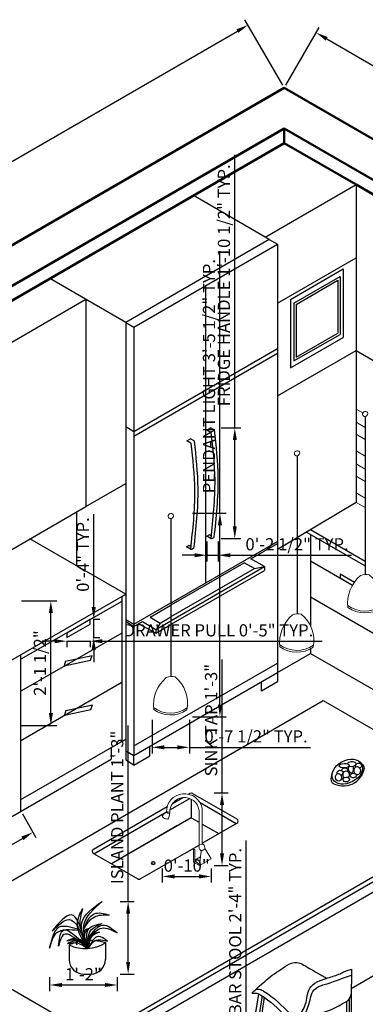
# Model space of a CAD drawing. Units: inches. Extents: x 5770 to 11891, y 3254 to 6808.
# Tile 3 of 15: x 5905 to 5976, y 3361 to 3563. Entities that reach past the tile are written whole.
import ezdxf

# ---------------------------------------------------------------- set-up
doc = ezdxf.new("R2010")
doc.units = ezdxf.units.IN
for name, color, linetype, lineweight in [('A-ANNO-DIMS', 2, 'Continuous', 18), ('A-FLOR-FIXT', 9, 'Continuous', 18), ('A-FURN', 8, 'Continuous', 25), ('A-WALL', 7, 'Continuous', 50), ('A-WALL-PATT', 8, 'Continuous', 13), ('E-LITE', 3, 'Continuous', 18)]:
    doc.layers.add(name, color=color, linetype=linetype, lineweight=lineweight)
doc.styles.get("Standard").update_dxf_attribs({"font": 'arial.ttf'})
doc.dimstyles.new('ISO-25', dxfattribs={"dimtxt": 2.5, "dimasz": 2.5, "dimexe": 1.25, "dimexo": 0.625, "dimtad": 1, "dimdec": 0, "dimlunit": 3, "dimtxsty": 'Standard', "dimcen": 2.5, "dimadec": 0, "dimazin": 0, "dimtfac": 1, "dimtdec": 0, "dimtmove": 0, "dimatfit": 3, "dimfxl": 1, "dimarcsym": 0})

# ---------------------------------------------------------------- blocks, each defined once
blk = doc.blocks.new('*D4')
at = {"layer": 'A-ANNO-DIMS', "color": 0, "lineweight": -2, "transparency": 16777216}
for p, q in [((5905.64, 3400.14), (5908.43, 3395.3)), ((5884.29, 3382.81), (5905.64, 3395.14)), ((5879.96, 3385.31), (5882.75, 3380.47))]:
    blk.add_line(p, q, dxfattribs=at)
at = {"layer": 'A-ANNO-DIMS', "color": 0, "transparency": 16777216}
for points in [[(5905.43, 3395.5), (5905.85, 3394.77), (5907.81, 3396.39)], [(5884.08, 3383.17), (5884.5, 3382.45), (5882.12, 3381.56)]]:
    blk.add_solid(points, dxfattribs=at)
at = {"layer": 'Defpoints', "color": 0, "transparency": 16777216}
for p in [(5905.33, 3400.68), (5907.81, 3396.39), (5879.65, 3385.85)]:
    blk.add_point(p, dxfattribs=at)
at = {"layer": 'A-ANNO-DIMS', "color": 0, "transparency": 16777216, "insert": (5894.02, 3390.62), "char_height": 2.5, "attachment_point": 5, "rotation": 30}
blk.add_mtext('2\'-6"', dxfattribs=at)
blk = doc.blocks.new('*D5')
at = {"layer": 'A-ANNO-DIMS', "color": 0, "lineweight": -2, "transparency": 16777216}
for p, q in [((5959, 3549.37), (5951.25, 3562.79)), ((5780.84, 3462.96), (5949.71, 3560.46)), ((5785.8, 3449.37), (5778.05, 3462.79))]:
    blk.add_line(p, q, dxfattribs=at)
at = {"layer": 'A-ANNO-DIMS', "color": 0, "transparency": 16777216}
for points in [[(5949.5, 3560.82), (5949.92, 3560.1), (5951.88, 3561.71)], [(5780.63, 3463.32), (5781.05, 3462.6), (5778.67, 3461.71)]]:
    blk.add_solid(points, dxfattribs=at)
at = {"layer": 'Defpoints', "color": 0, "transparency": 16777216}
for p in [(5951.88, 3561.71), (5959.31, 3548.83), (5786.11, 3448.83)]:
    blk.add_point(p, dxfattribs=at)
at = {"layer": 'A-ANNO-DIMS', "color": 0, "transparency": 16777216, "insert": (5864.32, 3513.36), "char_height": 2.5, "attachment_point": 5, "rotation": 30}
blk.add_mtext('16\'-8"', dxfattribs=at)
blk = doc.blocks.new('*D7')
at = {"layer": 'A-ANNO-DIMS', "color": 0, "lineweight": -2, "transparency": 16777216}
for p, q in [((5959.63, 3549.37), (5966.46, 3561.21)), ((5968, 3558.88), (6136.88, 3461.38)), ((6132.83, 3449.37), (6139.67, 3461.21))]:
    blk.add_line(p, q, dxfattribs=at)
at = {"layer": 'A-ANNO-DIMS', "color": 0, "transparency": 16777216}
for points in [[(5968.21, 3559.24), (5967.79, 3558.51), (5965.84, 3560.13)], [(6137.08, 3461.74), (6136.67, 3461.01), (6139.04, 3460.13)]]:
    blk.add_solid(points, dxfattribs=at)
at = {"layer": 'Defpoints', "color": 0, "transparency": 16777216}
for p in [(5959.31, 3548.83), (6139.04, 3460.13), (6132.52, 3448.83)]:
    blk.add_point(p, dxfattribs=at)
at = {"layer": 'A-ANNO-DIMS', "color": 0, "transparency": 16777216, "insert": (6061.62, 3507.02), "char_height": 2.5, "attachment_point": 5, "rotation": 330}
blk.add_mtext('16\'-8"', dxfattribs=at)
blk = doc.blocks.new('BULB')
for p, q in [((5936.06, 3465.13), (5936.06, 3432.77)), ((5936.16, 3465.15), (5936.16, 3432.77)), ((5936.06, 3432.77), (5936.16, 3432.77))]:
    blk.add_line(p, q)
for centre, radius, start, end in [((5939.83, 3426.9), 7.34, 129.7305, 187.2511), ((5936.2, 3430.31), 2.47, 73.0296, 115.4036), ((5932.63, 3427.32), 6.86, 348.0802, 51.2884), ((5936.01, 3431.26), 5.99, 234.2354, 304.5754), ((5935.99, 3430.88), 5.99, 234.9311, 303.9006)]:
    blk.add_arc(centre, radius, start, end)
blk.add_ellipse((5936.06, 3465.64), major_axis=(-0.492, -0.284), ratio=0.878374)
blk = doc.blocks.new('CHAIR')
for p, q in [((5928.22, 3348.4), (5925.54, 3331.45)), ((5928.97, 3347.97), (5926.27, 3331.03)), ((5929.39, 3347.7), (5926.87, 3331.3)), ((5946.78, 3347.31), (5946.81, 3331.7)), ((5947.21, 3348.3), (5947.24, 3331.95)), ((5946.25, 3346.87), (5946.28, 3331.94)), ((5935.16, 3343.21), (5935.19, 3327.16)), ((5935.65, 3343.13), (5935.69, 3326.87)), ((5936.61, 3343.23), (5936.64, 3327.43)), ((5936.93, 3343.31), (5936.93, 3335.67)), ((5937.63, 3343.48), (5937.63, 3336.08)), ((5927.75, 3337.02), (5935.16, 3341.28)), ((5937.62, 3341.89), (5946.27, 3336.9)), ((5937.62, 3341.39), (5946.27, 3336.4)), ((5927.68, 3336.56), (5935.16, 3340.78)), ((5935.18, 3331.68), (5927.6, 3336.05)), ((5935.18, 3332.18), (5927.67, 3336.51)), ((5936.63, 3335.85), (5936.93, 3335.67)), ((5946.27, 3336.9), (5936.64, 3331.34)), ((5946.27, 3336.4), (5936.64, 3330.84)), ((5937.63, 3336.08), (5936.93, 3335.67)), ((5925.54, 3331.45), (5926.27, 3331.03)), ((5926.27, 3331.03), (5926.87, 3331.3)), ((5946.28, 3331.94), (5946.75, 3331.67)), ((5946.75, 3331.67), (5947.24, 3331.95)), ((5935.69, 3326.87), (5935.19, 3327.16)), ((5935.69, 3326.87), (5936.64, 3327.43))]:
    blk.add_line(p, q)
blk.add_arc((5935.85, 3351.36), 3.39, 67.7359, 118.7768)
for points, knots in [([(5926.85, 3348.57), (5927.14, 3348.84), (5927.44, 3349.11), (5927.74, 3349.38), (5928.67, 3350.23), (5930.69, 3352.07), (5932.98, 3353.56), (5934.22, 3354.33)], [-1.200535, -1.200535, -1.200535, -1.200535, 0, 0, 0, 3.797995, 8.17369, 8.17369, 8.17369, 8.17369]), ([(5937.14, 3354.49), (5938.17, 3353.9), (5939.86, 3352.92), (5941.54, 3351.95), (5942.19, 3351.57)], [1.567957, 1.567957, 1.567957, 1.567957, 5.157778, 7.408601, 7.408601, 7.408601, 7.408601]), ([(5940.89, 3351.1), (5941.41, 3351.3), (5942.76, 3351.79), (5944.67, 3352.3), (5946.17, 3353.17), (5946.99, 3353.38), (5947.3, 3353.46)], [0, 0, 0, 0, 1.664278, 4.310629, 5.889247, 6.833724, 6.833724, 6.833724, 6.833724]), ([(5947.3, 3353.46), (5947.28, 3352.49), (5947.26, 3351.53), (5947.25, 3350.57), (5947.24, 3350.2), (5947.23, 3349.82), (5947.23, 3349.45), (5947.22, 3349.07), (5947.21, 3348.69), (5947.21, 3348.3)], [0, 0, 0, 0, 2.886502, 2.886502, 2.886502, 4.003886, 4.003886, 4.003886, 5.15459, 5.15459, 5.15459, 5.15459]), ([(5934.12, 3343.4), (5934.38, 3343.35), (5934.65, 3343.3), (5934.92, 3343.25), (5935.52, 3343.14), (5936.61, 3342.93), (5938.16, 3344.68), (5938.85, 3347.35), (5939.3, 3349.5), (5941.12, 3350.13), (5941.47, 3350.25), (5941.87, 3350.35), (5942.28, 3350.46), (5944.02, 3351.01), (5945.63, 3351.73), (5947.28, 3352.25)], [-0.758098, -0.758098, -0.758098, -0.758098, 0, 0, 0, 1.699756, 3.089131, 6.324639, 10.056959, 10.056959, 10.056959, 10.772274, 10.772274, 10.772274, 13.697346, 13.697346, 13.697346, 13.697346]), ([(5927.74, 3349.38), (5928, 3349.38), (5928.54, 3349.38), (5931.15, 3347.89), (5933.07, 3346.01), (5934.69, 3344.22)], [0, 0, 0, 0, 0.763361, 1.613257, 8.813397, 8.813397, 8.813397, 8.813397]), ([(5934.69, 3344.22), (5935.29, 3344.11), (5936.38, 3343.91), (5937.93, 3345.66), (5938.13, 3348.59), (5939.07, 3350.47), (5940.89, 3351.1)], [0, 0, 0, 0, 1.699756, 3.089131, 6.324639, 10.056959, 10.056959, 10.056959, 10.056959]), ([(5926.85, 3348.57), (5926.95, 3348.57), (5927.05, 3348.57), (5927.15, 3348.57), (5927.4, 3348.57), (5927.95, 3348.58), (5930.42, 3347.16), (5932.26, 3345.42), (5933.78, 3343.76), (5933.78, 3343.76), (5933.79, 3343.75), (5933.79, 3343.75), (5933.9, 3343.63), (5934.01, 3343.51), (5934.12, 3343.4)], [-0.293735, -0.293735, -0.293735, -0.293735, 0, 0, 0, 0.763361, 1.613257, 8.34273, 8.34273, 8.34273, 8.363036, 8.363036, 8.363036, 8.838355, 8.838355, 8.838355, 8.838355]), ([(5946.61, 3347.1), (5946.8, 3347.33), (5947.08, 3347.7), (5947.18, 3348.14), (5947.21, 3348.3)], [0, 0, 0, 0, 0.871891, 1.360739, 1.360739, 1.360739, 1.360739]), ([(5936.62, 3343.23), (5938.95, 3343.8), (5942.47, 3344.66), (5945.58, 3346.46), (5946.61, 3347.1)], [0, 0, 0, 0, 7.14919, 10.770772, 10.770772, 10.770772, 10.770772])]:
    blk.add_open_spline(points, degree=3, knots=knots)
blk = doc.blocks.new('TRESSS')
for p, q in [((5918.96, 3379.77), (5918.96, 3376.79)), ((5926.38, 3380.23), (5926.38, 3376.79)), ((5921.96, 3373.79), (5923.38, 3373.79))]:
    blk.add_line(p, q)
for centre, radius, start, end in [((5922.25, 3386.77), 7.74, 244.7929, 302.2014), ((5923.32, 3369.33), 11.31, 105.7826, 112.667), ((5923.32, 3369.33), 11.31, 101.3715, 102.257), ((5923.32, 3369.33), 11.31, 97.2364, 100.0777), ((5923.32, 3369.33), 11.31, 95.7662, 96.2014), ((5923.32, 3369.33), 11.31, 93.4301, 94.7766), ((5923.32, 3369.33), 11.31, 91.9955, 92.4941), ((5923.32, 3369.33), 11.31, 87.7241, 90.8189), ((5923.32, 3369.33), 11.31, 74.3273, 85.6124), ((5921.96, 3376.79), 3, 180, 270), ((5923.38, 3376.79), 3, 270, 0)]:
    blk.add_arc(centre, radius, start, end)
for points, knots in [([(5922.88, 3379.24), (5922.06, 3381.02), (5920.29, 3384.86), (5923.81, 3387.34), (5925.71, 3388.67)], [0, 0, 0, 0, 5.212698, 11.249377, 11.249377, 11.249377, 11.249377]), ([(5922.91, 3379.07), (5922.32, 3380.72), (5920.97, 3384.45), (5924.01, 3387.16), (5925.71, 3388.67)], [0, 0, 0, 0, 4.839765, 10.954456, 10.954456, 10.954456, 10.954456]), ([(5922.24, 3380.03), (5921.48, 3382.94), (5920.14, 3388.11), (5916.88, 3384.3), (5915.46, 3382.64)], [0, 0, 0, 0, 6.552433, 11.64556, 11.64556, 11.64556, 11.64556]), ([(5922.91, 3379.07), (5921.72, 3380.76), (5919.84, 3383.44), (5921.22, 3386.24), (5921.72, 3387.26)], [0, 0, 0, 0, 5.617277, 8.85563, 8.85563, 8.85563, 8.85563]), ([(5921.72, 3387.26), (5921.48, 3386.43), (5920.66, 3383.65), (5921.98, 3380.96), (5922.91, 3379.07)], [0, 0, 0, 0, 2.537454, 8.507618, 8.507618, 8.507618, 8.507618]), ([(5921.92, 3382.97), (5922.48, 3384.35), (5923.51, 3386.85), (5926.04, 3386.21), (5927.18, 3385.92)], [0, 0, 0, 0, 3.839673, 6.955686, 6.955686, 6.955686, 6.955686]), ([(5921.92, 3382.97), (5922.54, 3383.98), (5923.76, 3385.95), (5926.07, 3385.95), (5927.21, 3385.95)], [0, 0, 0, 0, 3.288518, 6.475213, 6.475213, 6.475213, 6.475213]), ([(5920.76, 3382.98), (5919.3, 3383.41), (5916.09, 3384.35), (5915.36, 3380.97), (5914.96, 3379.13)], [0, 0, 0, 0, 3.883772, 8.550412, 8.550412, 8.550412, 8.550412]), ([(5915.46, 3382.64), (5916.71, 3383.81), (5919.72, 3386.62), (5921.31, 3382.46), (5922.24, 3380.03)], [0, 0, 0, 0, 4.185411, 10.092894, 10.092894, 10.092894, 10.092894]), ([(5916.79, 3379.52), (5916.94, 3380.81), (5917.37, 3384.72), (5920.69, 3381.33), (5922.91, 3379.07)], [0, 0, 0, 0, 3.163863, 9.594114, 9.594114, 9.594114, 9.594114]), ([(5922.91, 3379.07), (5922.6, 3380.67), (5922.08, 3383.42), (5924.67, 3383.94), (5925.75, 3384.16)], [0, 0, 0, 0, 4.062167, 6.948759, 6.948759, 6.948759, 6.948759]), ([(5922.91, 3379.07), (5922.8, 3380.43), (5922.61, 3382.85), (5924.79, 3383.76), (5925.75, 3384.16)], [0, 0, 0, 0, 3.635219, 6.466255, 6.466255, 6.466255, 6.466255]), ([(5922.84, 3381.05), (5923.79, 3382.41), (5925.51, 3384.89), (5927.79, 3383.08), (5928.82, 3382.27)], [0, 0, 0, 0, 4.102984, 7.457094, 7.457094, 7.457094, 7.457094]), ([(5914.96, 3379.13), (5915.31, 3380.38), (5916.1, 3383.22), (5919.13, 3382.94), (5920.82, 3382.78)], [0, 0, 0, 0, 3.485265, 7.886828, 7.886828, 7.886828, 7.886828]), ([(5922.91, 3379.07), (5922.38, 3379.46), (5920.92, 3380.53), (5917.69, 3383.1), (5917.06, 3380.58), (5916.79, 3379.52)], [0, 0, 0, 0, 2.120674, 5.789324, 8.421631, 8.421631, 8.421631, 8.421631]), ([(5922.12, 3381.54), (5922.06, 3382.04), (5921.96, 3382.93), (5922.8, 3383.14), (5923.16, 3383.23)], [0, 0, 0, 0, 1.291281, 2.286027, 2.286027, 2.286027, 2.286027]), ([(5922.12, 3381.54), (5922.16, 3381.86), (5922.24, 3382.56), (5922.82, 3382.98), (5923.13, 3383.21)], [0, 0, 0, 0, 0.924204, 2.027617, 2.027617, 2.027617, 2.027617]), ([(5922.83, 3379.73), (5922.89, 3380.49), (5923, 3381.98), (5924.46, 3382.25), (5925.18, 3382.38)], [0, 0, 0, 0, 2.030096, 3.981846, 3.981846, 3.981846, 3.981846]), ([(5922.84, 3381.05), (5923.74, 3382.06), (5925.45, 3383.98), (5927.73, 3382.82), (5928.82, 3382.27)], [0, 0, 0, 0, 3.572941, 6.853548, 6.853548, 6.853548, 6.853548]), ([(5925.18, 3382.38), (5924.62, 3382.18), (5923.17, 3381.66), (5923.01, 3380.06), (5922.91, 3379.07)], [0, 0, 0, 0, 1.667038, 4.343126, 4.343126, 4.343126, 4.343126]), ([(5926.85, 3380.54), (5926.17, 3381.04), (5924.49, 3382.28), (5923.5, 3380.26), (5922.91, 3379.07)], [0, 0, 0, 0, 2.158738, 5.324445, 5.324445, 5.324445, 5.324445]), ([(5922.91, 3379.07), (5921.86, 3380.12), (5920.47, 3381.51), (5918.89, 3380.76), (5918.5, 3380.58)], [0, 0, 0, 0, 3.794821, 5.006614, 5.006614, 5.006614, 5.006614]), ([(5918.5, 3380.58), (5919.08, 3380.73), (5920.75, 3381.19), (5922.06, 3379.91), (5922.91, 3379.07)], [0, 0, 0, 0, 1.705074, 4.953728, 4.953728, 4.953728, 4.953728]), ([(5922.88, 3379.24), (5921.84, 3379.97), (5920.43, 3380.97), (5919.01, 3380.24), (5918.63, 3380.04)], [0, 0, 0, 0, 3.345341, 4.589329, 4.589329, 4.589329, 4.589329]), ([(5918.63, 3380.04), (5919.18, 3380.16), (5920.66, 3380.46), (5921.93, 3379.59), (5922.73, 3379.05)], [0, 0, 0, 0, 1.657681, 4.37303, 4.37303, 4.37303, 4.37303]), ([(5921.77, 3380.76), (5921.25, 3380.8), (5920.39, 3380.88), (5920.47, 3380.09), (5920.51, 3379.78)], [0, 0, 0, 0, 1.233849, 2.023752, 2.023752, 2.023752, 2.023752]), ([(5920.51, 3379.78), (5920.55, 3380.07), (5920.64, 3380.75), (5921.36, 3380.75), (5921.77, 3380.76)], [0, 0, 0, 0, 0.771667, 1.829769, 1.829769, 1.829769, 1.829769]), ([(5922.91, 3379.07), (5923.3, 3379.71), (5924.18, 3381.18), (5925.9, 3380.77), (5926.85, 3380.54)], [0, 0, 0, 0, 2.068412, 4.678786, 4.678786, 4.678786, 4.678786])]:
    blk.add_open_spline(points, degree=3, knots=knots)
blk = doc.blocks.new('*U16')
blk.add_circle((0, 0), 0.0159)
blk = doc.blocks.new('*U17')
at = {"layer": 'A-FURN', "color": 0, "linetype": 'ByBlock', "lineweight": -2, "transparency": 16777216}
for p, rotation in [((5932.23, 3390.22), 60), ((5932.24, 3389.96), 120), ((5932.47, 3389.82), 180), ((5932.7, 3390.23), 300), ((5932.7, 3389.96), 240)]:
    blk.add_blockref('*U16', p, dxfattribs=dict(at, rotation=rotation))
blk.add_blockref('*U16', (5932.47, 3390.36), dxfattribs=at)
blk = doc.blocks.new('TAP')
for p, q in [((5944.63, 3392.4), (5944.63, 3399.73)), ((5945.29, 3392.74), (5945.29, 3400.08)), ((5943.52, 3391.55), (5943.52, 3389.04)), ((5943.74, 3391.55), (5943.74, 3389.31)), ((5945.92, 3391.77), (5945.06, 3391.28)), ((5947.11, 3389.71), (5945.92, 3391.77)), ((5943.74, 3389.47), (5944.93, 3390.16)), ((5944.74, 3388.34), (5945.06, 3391.28)), ((5944.74, 3388.34), (5947.11, 3389.71)), ((5943.52, 3389.04), (5944.74, 3388.34)), ((5943.74, 3389.31), (5944.74, 3388.53))]:
    blk.add_line(p, q)
for centre, radius, start, end in [((5941.65, 3399.35), 3.7, 11.3324, 180.9911), ((5941.64, 3399.27), 3.02, 8.7526, 183.9319), ((5943.63, 3391.55), 0.111, 0, 180)]:
    blk.add_arc(centre, radius, start, end)
blk.add_ellipse((5938.29, 3399.19), major_axis=(-0.334, 0.124), ratio=0.36367)
for points, knots in [([(5937.95, 3399.3), (5937.78, 3399.2), (5937.42, 3399), (5937.21, 3398.66), (5937.11, 3398.48)], [0, 0, 0, 0, 0.588521, 1.1885, 1.1885, 1.1885, 1.1885]), ([(5937.11, 3398.48), (5937.18, 3398.34), (5937.38, 3397.9), (5937.89, 3397.88), (5938.22, 3397.87)], [0, 0, 0, 0, 0.468589, 1.360834, 1.360834, 1.360834, 1.360834]), ([(5938.63, 3399.07), (5938.6, 3398.79), (5938.56, 3398.35), (5938.31, 3398), (5938.22, 3397.87)], [0, 0, 0, 0, 0.813794, 1.27848, 1.27848, 1.27848, 1.27848]), ([(5945.06, 3391.28), (5944.95, 3391.43), (5944.74, 3391.76), (5944.43, 3392.52), (5945.18, 3392.82), (5945.66, 3392.65), (5945.72, 3392.21), (5945.85, 3391.92), (5945.92, 3391.77)], [0, 0, 0, 0, 0.574345, 1.207986, 2.06998, 2.194026, 2.686402, 3.17968, 3.17968, 3.17968, 3.17968])]:
    blk.add_open_spline(points, degree=3, knots=knots)
blk = doc.blocks.new('FRIDGE-HANDLE')
for p, q in [((0.04, 22.22), (0.8, 22.65)), ((0.87, 21.74), (0.04, 22.22)), ((1.53, 22.23), (0.8, 22.65)), ((0, 0.48), (0.52, 0.78)), ((0.82, 0), (0, 0.48)), ((0.88, 0.57), (0.52, 0.78))]:
    blk.add_line(p, q)
blk.add_arc((0.89, 0.84), 0.836, 265.562, 313.7192)
for points, knots in [([(1.53, 22.23), (1.89, 18.98), (2.7, 11.65), (1.91, 4.32), (1.47, 0.23)], [0, 0, 0, 0, 9.778963, 22.056344, 22.056344, 22.056344, 22.056344]), ([(0.87, 21.74), (1.23, 18.49), (2.03, 11.25), (1.25, 4), (0.82, 0)], [0, 0, 0, 0, 9.778963, 21.793888, 21.793888, 21.793888, 21.793888])]:
    blk.add_open_spline(points, degree=3, knots=knots)
blk = doc.blocks.new('DRAWER-PULL')
for p, q in [((0, 1), (4.81, 3.78)), ((0, 0), (4.81, 2.77)), ((4.81, 2.77), (4.81, 3.78)), ((0, 1), (0, 0))]:
    blk.add_line(p, q)
blk = doc.blocks.new('*D26')
at = {"layer": 'A-ANNO-DIMS', "color": 0, "lineweight": -2, "transparency": 16777216}
for p, q in [((5951.5, 3354.88), (5951.5, 3394.72)), ((5947.92, 3354.88), (5952.75, 3354.88)), ((5951.5, 3329.37), (5951.5, 3352.38)), ((5947.92, 3326.87), (5952.75, 3326.87))]:
    blk.add_line(p, q, dxfattribs=at)
at = {"layer": 'A-ANNO-DIMS', "color": 0, "transparency": 16777216}
for points in [[(5951.08, 3352.38), (5951.91, 3352.38), (5951.5, 3354.88)], [(5951.08, 3329.37), (5951.91, 3329.37), (5951.5, 3326.87)]]:
    blk.add_solid(points, dxfattribs=at)
at = {"layer": 'Defpoints', "color": 0, "transparency": 16777216}
for p in [(5947.3, 3354.88), (5951.5, 3354.88), (5947.3, 3326.87)]:
    blk.add_point(p, dxfattribs=at)
at = {"layer": 'A-ANNO-DIMS', "color": 0, "transparency": 16777216, "insert": (5949.58, 3376.05), "char_height": 2.5, "attachment_point": 5, "rotation": 90}
blk.add_mtext('BAR STOOL 2\'-4" TYP.', dxfattribs=at)
blk = doc.blocks.new('*D28')
at = {"layer": 'A-ANNO-DIMS', "color": 0, "lineweight": -2, "transparency": 16777216}
for p, q in [((5946.13, 3461.75), (5946.13, 3515.36)), ((5940.5, 3461.75), (5947.38, 3461.75)), ((5946.13, 3422.54), (5946.13, 3459.25)), ((5940.5, 3420.04), (5947.38, 3420.04))]:
    blk.add_line(p, q, dxfattribs=at)
at = {"layer": 'A-ANNO-DIMS', "color": 0, "transparency": 16777216}
for points in [[(5945.71, 3459.25), (5946.55, 3459.25), (5946.13, 3461.75)], [(5945.71, 3422.54), (5946.55, 3422.54), (5946.13, 3420.04)]]:
    blk.add_solid(points, dxfattribs=at)
at = {"layer": 'Defpoints', "color": 0, "transparency": 16777216}
for p in [(5939.87, 3461.75), (5946.13, 3461.75), (5939.87, 3420.04)]:
    blk.add_point(p, dxfattribs=at)
at = {"layer": 'A-ANNO-DIMS', "color": 0, "transparency": 16777216, "insert": (5944.21, 3489.8), "char_height": 2.5, "attachment_point": 5, "rotation": 90}
blk.add_mtext('PENDANT LIGHT 3\'-5 1/2" TYP.', dxfattribs=at)
blk = doc.blocks.new('*D29')
at = {"layer": 'A-ANNO-DIMS', "color": 0, "lineweight": -2, "transparency": 16777216}
for p, q in [((5932.23, 3419.41), (5932.23, 3412.53)), ((5939.87, 3419.41), (5939.87, 3412.53)), ((5934.73, 3413.78), (5937.37, 3413.78)), ((5939.87, 3413.78), (5964.69, 3413.78))]:
    blk.add_line(p, q, dxfattribs=at)
at = {"layer": 'A-ANNO-DIMS', "color": 0, "transparency": 16777216}
for points in [[(5934.73, 3414.2), (5934.73, 3413.36), (5932.23, 3413.78)], [(5937.37, 3414.2), (5937.37, 3413.36), (5939.87, 3413.78)]]:
    blk.add_solid(points, dxfattribs=at)
at = {"layer": 'Defpoints', "color": 0, "transparency": 16777216}
for p in [(5932.23, 3420.04), (5939.87, 3420.04), (5939.87, 3413.78)]:
    blk.add_point(p, dxfattribs=at)
at = {"layer": 'A-ANNO-DIMS', "color": 0, "transparency": 16777216, "insert": (5953.53, 3415.7), "char_height": 2.5, "attachment_point": 5}
blk.add_mtext('0\'-7 1/2" TYP.', dxfattribs=at)
blk = doc.blocks.new('*D31')
at = {"layer": 'A-ANNO-DIMS', "color": 0, "lineweight": -2, "transparency": 16777216}
for p, q in [((5905.48, 3443.8), (5912.73, 3443.8)), ((5911.48, 3420.78), (5911.48, 3441.3)), ((5905.48, 3418.28), (5912.73, 3418.28))]:
    blk.add_line(p, q, dxfattribs=at)
at = {"layer": 'A-ANNO-DIMS', "color": 0, "transparency": 16777216}
for points in [[(5911.07, 3441.3), (5911.9, 3441.3), (5911.48, 3443.8)], [(5911.07, 3420.78), (5911.9, 3420.78), (5911.48, 3418.28)]]:
    blk.add_solid(points, dxfattribs=at)
at = {"layer": 'Defpoints', "color": 0, "transparency": 16777216}
for p in [(5904.85, 3443.8), (5911.48, 3443.8), (5904.85, 3418.28)]:
    blk.add_point(p, dxfattribs=at)
at = {"layer": 'A-ANNO-DIMS', "color": 0, "transparency": 16777216, "insert": (5909.57, 3431.04), "char_height": 2.5, "attachment_point": 5, "rotation": 90}
blk.add_mtext('2\'-1 1/2"', dxfattribs=at)
blk = doc.blocks.new('*D32')
at = {"layer": 'A-ANNO-DIMS', "color": 0, "lineweight": -2, "transparency": 16777216}
for p, q in [((5946.56, 3404.47), (5946.56, 3431.74)), ((5944.95, 3404.47), (5947.81, 3404.47)), ((5946.56, 3392.07), (5946.56, 3401.97)), ((5944.95, 3389.57), (5947.81, 3389.57))]:
    blk.add_line(p, q, dxfattribs=at)
at = {"layer": 'A-ANNO-DIMS', "color": 0, "transparency": 16777216}
for points in [[(5946.14, 3401.97), (5946.97, 3401.97), (5946.56, 3404.47)], [(5946.14, 3392.07), (5946.97, 3392.07), (5946.56, 3389.57)]]:
    blk.add_solid(points, dxfattribs=at)
at = {"layer": 'Defpoints', "color": 0, "transparency": 16777216}
for p in [(5944.32, 3404.47), (5946.56, 3404.47), (5944.32, 3389.57)]:
    blk.add_point(p, dxfattribs=at)
at = {"layer": 'A-ANNO-DIMS', "color": 0, "transparency": 16777216, "insert": (5944.64, 3419.35), "char_height": 2.5, "attachment_point": 5, "rotation": 90}
blk.add_mtext('SINK TAP 1\'-3"', dxfattribs=at)
blk = doc.blocks.new('*D33')
at = {"layer": 'A-ANNO-DIMS', "color": 0, "lineweight": -2, "transparency": 16777216}
for p, q in [((5934.32, 3388.95), (5934.32, 3386.09)), ((5944.32, 3388.95), (5944.32, 3386.09)), ((5936.82, 3387.34), (5941.82, 3387.34))]:
    blk.add_line(p, q, dxfattribs=at)
at = {"layer": 'A-ANNO-DIMS', "color": 0, "transparency": 16777216}
for points in [[(5936.82, 3387.76), (5936.82, 3386.92), (5934.32, 3387.34)], [(5941.82, 3387.76), (5941.82, 3386.92), (5944.32, 3387.34)]]:
    blk.add_solid(points, dxfattribs=at)
at = {"layer": 'Defpoints', "color": 0, "transparency": 16777216}
for p in [(5934.32, 3389.57), (5944.32, 3389.57), (5944.32, 3387.34)]:
    blk.add_point(p, dxfattribs=at)
at = {"layer": 'A-ANNO-DIMS', "color": 0, "transparency": 16777216, "insert": (5939.32, 3389.24), "char_height": 2.5, "attachment_point": 5}
blk.add_mtext('0\'-10"', dxfattribs=at)
blk = doc.blocks.new('*D34')
at = {"layer": 'A-ANNO-DIMS', "color": 0, "lineweight": -2, "transparency": 16777216}
for p, q in [((5949.17, 3479.19), (5949.17, 3535.11)), ((5946.4, 3479.19), (5950.42, 3479.19)), ((5949.17, 3459.02), (5949.17, 3476.69)), ((5946.4, 3456.52), (5950.42, 3456.52))]:
    blk.add_line(p, q, dxfattribs=at)
at = {"layer": 'A-ANNO-DIMS', "color": 0, "transparency": 16777216}
for points in [[(5948.76, 3476.69), (5949.59, 3476.69), (5949.17, 3479.19)], [(5948.76, 3459.02), (5949.59, 3459.02), (5949.17, 3456.52)]]:
    blk.add_solid(points, dxfattribs=at)
at = {"layer": 'Defpoints', "color": 0, "transparency": 16777216}
for p in [(5945.77, 3479.19), (5949.17, 3479.19), (5945.77, 3456.52)]:
    blk.add_point(p, dxfattribs=at)
at = {"layer": 'A-ANNO-DIMS', "color": 0, "transparency": 16777216, "insert": (5947.26, 3508.4), "char_height": 2.5, "attachment_point": 5, "rotation": 90}
blk.add_mtext('FRIDGE HANDLE 1\'-10 1/2" TYP.', dxfattribs=at)
blk = doc.blocks.new('*D35')
at = {"layer": 'A-ANNO-DIMS', "color": 0, "lineweight": -2, "transparency": 16777216}
for p, q in [((5943.42, 3455.9), (5943.42, 3451.87)), ((5945.77, 3455.9), (5945.77, 3451.87)), ((5940.92, 3453.12), (5938.42, 3453.12)), ((5943.42, 3453.12), (5945.77, 3453.12)), ((5948.27, 3453.12), (5973.09, 3453.12))]:
    blk.add_line(p, q, dxfattribs=at)
at = {"layer": 'A-ANNO-DIMS', "color": 0, "transparency": 16777216}
for points in [[(5940.92, 3453.54), (5940.92, 3452.7), (5943.42, 3453.12)], [(5948.27, 3453.54), (5948.27, 3452.7), (5945.77, 3453.12)]]:
    blk.add_solid(points, dxfattribs=at)
at = {"layer": 'Defpoints', "color": 0, "transparency": 16777216}
for p in [(5943.42, 3456.52), (5945.77, 3456.52), (5945.77, 3453.12)]:
    blk.add_point(p, dxfattribs=at)
at = {"layer": 'A-ANNO-DIMS', "color": 0, "transparency": 16777216, "insert": (5961.93, 3455.04), "char_height": 2.5, "attachment_point": 5}
blk.add_mtext('0\'-2 1/2" TYP.', dxfattribs=at)
blk = doc.blocks.new('*D36')
at = {"layer": 'A-ANNO-DIMS', "color": 0, "lineweight": -2, "transparency": 16777216}
for p, q in [((5912.23, 3435.52), (5909.73, 3435.52)), ((5914.73, 3435.61), (5914.73, 3434.27)), ((5914.73, 3435.52), (5919.54, 3435.52)), ((5919.54, 3435.61), (5919.54, 3434.27)), ((5922.04, 3435.52), (5967.1, 3435.52))]:
    blk.add_line(p, q, dxfattribs=at)
at = {"layer": 'A-ANNO-DIMS', "color": 0, "transparency": 16777216}
for points in [[(5912.23, 3435.93), (5912.23, 3435.1), (5914.73, 3435.52)], [(5922.04, 3435.93), (5922.04, 3435.1), (5919.54, 3435.52)]]:
    blk.add_solid(points, dxfattribs=at)
at = {"layer": 'Defpoints', "color": 0, "transparency": 16777216}
for p in [(5914.73, 3436.24), (5919.54, 3436.24), (5919.54, 3435.52)]:
    blk.add_point(p, dxfattribs=at)
at = {"layer": 'A-ANNO-DIMS', "color": 0, "transparency": 16777216, "insert": (5945.82, 3437.42), "char_height": 2.5, "attachment_point": 5}
blk.add_mtext('DRAWER PULL 0\'-5" TYP.', dxfattribs=at)
blk = doc.blocks.new('*D37')
at = {"layer": 'A-ANNO-DIMS', "color": 0, "lineweight": -2, "transparency": 16777216}
for p, q in [((5920.26, 3442.51), (5920.26, 3461.5)), ((5920.16, 3440.01), (5921.51, 3440.01)), ((5920.26, 3436.24), (5920.26, 3440.01)), ((5920.16, 3436.24), (5921.51, 3436.24)), ((5920.26, 3433.74), (5920.26, 3431.24))]:
    blk.add_line(p, q, dxfattribs=at)
at = {"layer": 'A-ANNO-DIMS', "color": 0, "transparency": 16777216}
for points in [[(5919.84, 3442.51), (5920.68, 3442.51), (5920.26, 3440.01)], [(5919.84, 3433.74), (5920.68, 3433.74), (5920.26, 3436.24)]]:
    blk.add_solid(points, dxfattribs=at)
at = {"layer": 'Defpoints', "color": 0, "transparency": 16777216}
for p in [(5919.54, 3440.01), (5920.26, 3440.01), (5919.54, 3436.24)]:
    blk.add_point(p, dxfattribs=at)
at = {"layer": 'A-ANNO-DIMS', "color": 0, "transparency": 16777216, "insert": (5918.36, 3453.26), "char_height": 2.5, "attachment_point": 5, "rotation": 90}
blk.add_mtext('0\'-4" TYP.', dxfattribs=at)
blk = doc.blocks.new('*D40')
at = {"layer": 'A-ANNO-DIMS', "color": 0, "lineweight": -2, "transparency": 16777216}
for p, q in [((5927.32, 3382.22), (5927.32, 3418.25)), ((5925.71, 3382.22), (5928.57, 3382.22)), ((5927.32, 3369.84), (5927.32, 3379.72)), ((5925.71, 3367.34), (5928.57, 3367.34))]:
    blk.add_line(p, q, dxfattribs=at)
at = {"layer": 'A-ANNO-DIMS', "color": 0, "transparency": 16777216}
for points in [[(5926.9, 3379.72), (5927.73, 3379.72), (5927.32, 3382.22)], [(5926.9, 3369.84), (5927.73, 3369.84), (5927.32, 3367.34)]]:
    blk.add_solid(points, dxfattribs=at)
at = {"layer": 'Defpoints', "color": 0, "transparency": 16777216}
for p in [(5925.09, 3382.22), (5927.32, 3382.22), (5925.09, 3367.34)]:
    blk.add_point(p, dxfattribs=at)
at = {"layer": 'A-ANNO-DIMS', "color": 0, "transparency": 16777216, "insert": (5925.4, 3401.48), "char_height": 2.5, "attachment_point": 5, "rotation": 90}
blk.add_mtext('ISLAND PLANT 1\'-3"', dxfattribs=at)
blk = doc.blocks.new('*D41')
at = {"layer": 'A-ANNO-DIMS', "color": 0, "lineweight": -2, "transparency": 16777216}
for p, q in [((5911.23, 3366.72), (5911.23, 3363.86)), ((5925.09, 3366.72), (5925.09, 3363.86)), ((5913.73, 3365.11), (5922.59, 3365.11))]:
    blk.add_line(p, q, dxfattribs=at)
at = {"layer": 'A-ANNO-DIMS', "color": 0, "transparency": 16777216}
for points in [[(5913.73, 3365.53), (5913.73, 3364.7), (5911.23, 3365.11)], [(5922.59, 3365.53), (5922.59, 3364.7), (5925.09, 3365.11)]]:
    blk.add_solid(points, dxfattribs=at)
at = {"layer": 'Defpoints', "color": 0, "transparency": 16777216}
for p in [(5911.23, 3367.34), (5925.09, 3367.34), (5925.09, 3365.11)]:
    blk.add_point(p, dxfattribs=at)
at = {"layer": 'A-ANNO-DIMS', "color": 0, "transparency": 16777216, "insert": (5918.16, 3366.99), "char_height": 2.5, "attachment_point": 5}
blk.add_mtext('1\'-2"', dxfattribs=at)

msp = doc.modelspace()

# ---------------------------------------------------------------- linework, layer by layer
at = {"layer": 'A-FURN'}
for p, q in [((5955.4, 3518.27), (5974.02, 3529.02)), ((5974.02, 3529.02), (5974.02, 3463.94)), ((5956.22, 3517.8), (5940.69, 3526.76)), ((5956.22, 3517.8), (5926.81, 3500.81)), ((5928.51, 3499.83), (5957.92, 3516.81)), ((5956.22, 3517.8), (5957.92, 3516.81)), ((5957.92, 3516.81), (5957.92, 3429.08)), ((5957.92, 3504.75), (5974.02, 3514.05)), ((5974.02, 3513.28), (5974.02, 3499.24)), ((5960.56, 3505.52), (5971.38, 3511.77)), ((5971.38, 3511.77), (5971.38, 3497.72)), ((5926.81, 3500.81), (5911.28, 3509.78)), ((5961.3, 3504.75), (5970.74, 3510.2)), ((5961.74, 3504.5), (5970.31, 3509.45)), ((5970.31, 3509.45), (5970.31, 3498.6)), ((5970.74, 3510.2), (5970.74, 3498.35)), ((5943.21, 3447.47), (5943.21, 3508.32)), ((5891.5, 3489.87), (5918.64, 3505.53)), ((5918.64, 3505.53), (5918.64, 3463.08)), ((5960.56, 3505.52), (5960.56, 3491.47)), ((5961.3, 3504.75), (5961.3, 3492.91)), ((5961.74, 3504.5), (5961.74, 3493.66)), ((5926.81, 3500.81), (5926.81, 3466.85)), ((5926.81, 3500.81), (5928.51, 3499.83)), ((5928.51, 3499.83), (5928.51, 3412.1)), ((5961.74, 3493.66), (5970.31, 3498.6)), ((5960.56, 3491.47), (5971.38, 3497.72)), ((5961.3, 3492.91), (5970.74, 3498.35)), ((5928.51, 3478.48), (5957.92, 3495.46)), ((5928.51, 3477.53), (5957.92, 3494.51)), ((5957.92, 3485.76), (5974.02, 3495.06)), ((5957.92, 3485.76), (5974.02, 3495.06)), ((5974.02, 3495.06), (6002.6, 3478.56)), ((5926.81, 3479.5), (5928.51, 3478.48)), ((5918.64, 3463.08), (5926.81, 3467.8)), ((5926.81, 3466.85), (5926.81, 3413.08)), ((5898.94, 3451.71), (5918.64, 3463.08)), ((5974.02, 3463.94), (5962.03, 3456.76)), ((5916.76, 3462), (5916.76, 3450.95)), ((5964.71, 3458.36), (5975.87, 3451.92)), ((5926.81, 3445.15), (5907.2, 3456.47)), ((5961.93, 3456.7), (5957.92, 3454.3)), ((5963.86, 3457.85), (5975.87, 3450.92)), ((5964.71, 3457.36), (5964.71, 3438.59)), ((5936.16, 3443.4), (5957.92, 3455.96)), ((5952.49, 3452.38), (5957.92, 3455.51)), ((5955.23, 3450.79), (5952.49, 3452.38)), ((5936.16, 3442.95), (5951.12, 3451.58)), ((5936.16, 3439.78), (5955.23, 3450.79)), ((5936.16, 3440.57), (5953.18, 3450.39)), ((5936.16, 3438.98), (5955.23, 3449.99)), ((5953.18, 3450.39), (5951.12, 3451.58)), ((5953.18, 3450.39), (5955.23, 3450.79)), ((5955.23, 3450.79), (5955.23, 3449.99)), ((5964.71, 3451.98), (5973.3, 3447.02)), ((5964.71, 3451.98), (5973.3, 3447.02)), ((5970.77, 3449.3), (5973.69, 3447.62)), ((5970.77, 3449.3), (5970.77, 3448.48)), ((5970.77, 3449.3), (5970.77, 3448.48)), ((5970.77, 3448.48), (5973.3, 3447.02)), ((5815.52, 3380.9), (5925.99, 3444.68)), ((5925.99, 3444.68), (5926.81, 3445.15)), ((5925.99, 3444.68), (5926.81, 3445.15)), ((5925.99, 3444.68), (5925.99, 3415)), ((5964.71, 3444.58), (5986.36, 3432.08)), ((5925.99, 3443.67), (5905.33, 3431.81)), ((5928.51, 3438.98), (5936.06, 3443.34)), ((5931.8, 3440.43), (5936.06, 3442.89)), ((5926.81, 3439.97), (5928.51, 3438.98)), ((5931.8, 3440.43), (5933.86, 3439.24)), ((5933.86, 3439.24), (5936.06, 3440.51)), ((5926.81, 3439.52), (5928.51, 3438.53)), ((5928.51, 3438.53), (5930.23, 3439.53)), ((5932.98, 3437.14), (5929.42, 3439.06)), ((5930.23, 3439.53), (5932.98, 3437.94)), ((5932.98, 3437.94), (5936.06, 3439.72)), ((5932.98, 3437.14), (5936.06, 3438.92)), ((5932.98, 3437.94), (5932.98, 3437.14)), ((5933.86, 3439.24), (5933.18, 3438.06)), ((5925.99, 3437.18), (5905.33, 3425.25)), ((5964.71, 3433.97), (5964.71, 3433)), ((5905.33, 3400.68), (5905.33, 3432.75)), ((5957.92, 3429.08), (5964.71, 3433)), ((5964.71, 3433), (6059.32, 3378.37)), ((5928.51, 3414.06), (5957.92, 3431.04)), ((5928.51, 3412.1), (5957.92, 3429.08)), ((5957.92, 3429.08), (5957.92, 3427.19)), ((5925.99, 3427.03), (5905.33, 3415.1)), ((5957.92, 3427.19), (5954.65, 3425.3)), ((5954.65, 3425.3), (5954.65, 3427.19)), ((5884.12, 3375.37), (5967.26, 3423.37)), ((5967.26, 3423.37), (6003.63, 3402.37)), ((5905.33, 3403.07), (5926.81, 3415.47)), ((5923.86, 3413.77), (5923.86, 3411.38)), ((5931.78, 3412.01), (5931.78, 3413.98)), ((5926.81, 3413.08), (5928.51, 3412.1)), ((5926.81, 3413.08), (5926.81, 3411.19)), ((5928.51, 3410.21), (5928.51, 3412.1)), ((5928.51, 3410.12), (5931.78, 3412.01)), ((5881.06, 3386.67), (5923.86, 3411.38)), ((5926.81, 3411.19), (5928.51, 3410.21)), ((5939.7, 3404.19), (5939.99, 3404.36)), ((5940.49, 3404.36), (5949.58, 3399.11)), ((5920.2, 3392.93), (5935.32, 3401.66)), ((5920.5, 3354.37), (6003.63, 3402.37)), ((5935.86, 3400.98), (5939.94, 3403.33)), ((5936.41, 3402.29), (5938.52, 3403.51)), ((5940.24, 3403.19), (5940.24, 3399.37)), ((5942.06, 3402.45), (5949.47, 3398.17)), ((5920.32, 3392), (5935.16, 3400.57)), ((5921.36, 3353.87), (6002.77, 3400.87)), ((5940.24, 3399.37), (5923.9, 3389.93)), ((5937.32, 3397.68), (5923.9, 3389.93)), ((5940.24, 3399.37), (5941.84, 3398.44)), ((5942.49, 3394.15), (5949.58, 3398.24)), ((5942.49, 3398.06), (5945.88, 3396.11)), ((5922.46, 3352.37), (5996.03, 3394.84)), ((5938.85, 3392.04), (5941.84, 3393.77)), ((5920.2, 3392.07), (5929.3, 3386.82)), ((5929.8, 3386.82), (5938.85, 3392.04)), ((5920.5, 3354.37), (5884.12, 3375.37)), ((5978.2, 3367.34), (5973.04, 3364.35))]:
    msp.add_line(p, q, dxfattribs=at)
for radius in [0.343, 0.321]:
    msp.add_circle((5932.47, 3390.09), radius, dxfattribs=at)
for centre, radius, start, end in [((5974.84, 3409.53), 0.891, 0.7333, 69.1986), ((5970.24, 3407.38), 1.39, 145.2066, 218.1089), ((5971.42, 3410.23), 4.36, 238.3961, 350.9471), ((5940.24, 3403.92), 0.5, 60, 120), ((5949.33, 3398.67), 0.5, 300, 60), ((5920.45, 3392.5), 0.5, 120, 240), ((5929.55, 3387.25), 0.5, 240, 300)]:
    msp.add_arc(centre, radius, start, end, dxfattribs=at)
msp.add_ellipse((5972.22, 3408.79), major_axis=(-2.94, -1.56), ratio=0.693198, dxfattribs=at)
for centre, major_axis, ratio, start_param, end_param in [((5971.6, 3410.02), (1.01, 0.06), 0.460203, -1.570796, 4.712389), ((5973.13, 3410.35), (0.892, 0.049), 0.522988, 4.032458, 9.209641), ((5972.97, 3409.36), (-0.045, 0.824), 0.647718, 0.71797, 5.409531), ((5974.26, 3408.99), (-0.046, 0.85), 0.751507, -3.141592653589793, 3.141592653589793), ((5974.54, 3410.01), (0.639, 0.035), 0.729895, -1.332229, 3.617996), ((5970.43, 3407.62), (-0.043, 0.781), 0.817825, -3.141592653589793, 3.141592653589793), ((5970.73, 3408.55), (0.639, 0.035), 0.729895, -1.317272, 3.560326), ((5971.7, 3409.05), (0.639, 0.035), 0.729895, -0.484058, 3.267141), ((5972.01, 3407.18), (0.639, 0.035), 0.7713, -1.570796, 4.712389), ((5971.7, 3409.05), (0.639, 0.035), 0.729895, 4.106473, 4.284675), ((5973.45, 3408), (0.639, 0.035), 0.729895, -1.570796, 4.712389)]:
    msp.add_ellipse(centre, major_axis=major_axis, ratio=ratio, start_param=start_param, end_param=end_param, dxfattribs=at)
at = {"layer": 'A-FURN', "extrusion": (0, 0, -1)}
msp.add_ellipse((5972, 3408.16), major_axis=(0.043, -0.796), ratio=0.803016, start_param=0.73902, end_param=5.61046, dxfattribs=at)
at = {"layer": 'A-WALL'}
for p, q in [((5959.31, 3548.83), (5786.11, 3448.83)), ((5959.31, 3548.83), (6132.52, 3448.83)), ((5795.91, 3446.17), (5959.31, 3540.51)), ((5959.31, 3540.51), (6115.24, 3450.48)), ((5959.31, 3540.51), (5959.31, 3537.51)), ((5795.91, 3443.17), (5959.31, 3537.51)), ((5959.31, 3537.51), (5974.02, 3529.02)), ((5974.02, 3529.02), (6111.68, 3448.43))]:
    msp.add_line(p, q, dxfattribs=at)
at = {"layer": 'A-WALL-PATT'}
for p, q in [((5974.02, 3483.06), (5975.39, 3482.27)), ((5974.02, 3480.39), (5975.87, 3479.31)), ((5974.02, 3477.88), (5975.87, 3476.81)), ((5974.02, 3474.48), (5975.87, 3473.41)), ((5974.02, 3471.81), (5975.87, 3470.74)), ((5974.02, 3469.3), (5975.87, 3468.24)), ((5974.02, 3465.91), (5975.87, 3464.84)), ((5974.02, 3463.94), (5975.87, 3462.87))]:
    msp.add_line(p, q, dxfattribs=at)

# ---------------------------------------------------------------- block references
at = {"layer": 'A-FLOR-FIXT'}
msp.add_blockref('TAP', (-2.79, 1.23), dxfattribs=at)
at = {"layer": 'A-FURN'}
for name, p in [('FRIDGE-HANDLE', (5943.42, 3456.54)), ('DRAWER-PULL', (5914.73, 3436.24)), ('*U17', (0, 0)), ('TRESSS', (-3.73, -6.45)), ('CHAIR', (25.81, 14.9))]:
    msp.add_blockref(name, p, dxfattribs=at)
for name, p, rotation in [('FRIDGE-HANDLE', (5939.26, 3454.34), 359.8707584858055), ('DRAWER-PULL', (5914.2, 3430.47), 342.0601581916923), ('DRAWER-PULL', (5914.26, 3420.36), 342.0601581916947)]:
    msp.add_blockref(name, p, dxfattribs=dict(at, rotation=rotation))
at = {"layer": 'E-LITE'}
for p in [(39.81, 16.42), (25.87, 8.37), (0, -4.48)]:
    msp.add_blockref('BULB', p, dxfattribs=at)

# ---------------------------------------------------------------- dimensions: what is measured, and where the dimension line sits
at = {"layer": 'A-ANNO-DIMS'}
for p1, p2, distance, picture, middle in [((5786.11, 3448.83), (5959.31, 3548.83), 14.87, '*D5', (5864.32, 3513.36)), ((5879.65, 3385.85), (5905.33, 3400.68), -4.96, '*D4', (5894.02, 3390.62))]:
    dim = msp.add_aligned_dim(p1=p1, p2=p2, distance=distance, dimstyle='ISO-25', override={"dimclrd": 0, "dimclre": 0, "dimclrt": 0}, dxfattribs=at)
    dim.commit()
    dim.dimension.update_dxf_attribs({"geometry": picture, "text_midpoint": middle})
dim = msp.add_linear_dim(base=(6139.04, 3460.13), p1=(5959.31, 3548.83), p2=(6132.52, 3448.83), angle=330, dimstyle='ISO-25', override={"dimclrd": 0, "dimclre": 0, "dimclrt": 0}, dxfattribs=at)
dim.commit()
dim.dimension.update_dxf_attribs({"geometry": '*D7', "text_midpoint": (6060.67, 3505.37), "dimtype": 161})
for base, p1, p2, text, picture, middle in [((5949.17, 3479.19), (5945.77, 3456.52), (5945.77, 3479.19), 'FRIDGE HANDLE <> TYP.', '*D34', (5947.26, 3508.4)), ((5946.13, 3461.75), (5939.87, 3420.04), (5939.87, 3461.75), 'PENDANT LIGHT <> TYP.', '*D28', (5944.21, 3489.8)), ((5920.26, 3440.01), (5919.54, 3436.24), (5919.54, 3440.01), '<> TYP.', '*D37', (5918.36, 3453.26)), ((5946.56, 3404.47), (5944.32, 3389.57), (5944.32, 3404.47), 'SINK TAP <>', '*D32', (5944.64, 3419.35)), ((5927.32, 3382.22), (5925.09, 3367.34), (5925.09, 3382.22), 'ISLAND PLANT <>', '*D40', (5925.4, 3401.48)), ((5951.5, 3354.88), (5947.3, 3326.87), (5947.3, 3354.88), 'BAR STOOL <> TYP.', '*D26', (5949.58, 3376.05))]:
    dim = msp.add_linear_dim(base=base, p1=p1, p2=p2, angle=90, text=text, dimstyle='ISO-25', override={"dimdec": 1, "dimlfac": 1, "dimrnd": 0, "dimzin": 1, "dimdsep": 46, "dimlunit": 4, "dimfrac": 2}, dxfattribs=at)
    dim.commit()
    dim.dimension.update_dxf_attribs({"geometry": picture, "text_midpoint": middle})
for base, p1, p2, text, picture, middle in [((5945.774, 3453.1199), (5943.4233, 3456.5202), (5945.774, 3456.5202), '<> TYP.', '*D35', (5961.931, 3455.0376)), ((5919.54, 3435.52), (5914.73, 3436.24), (5919.54, 3436.24), 'DRAWER PULL <> TYP.', '*D36', (5945.82, 3437.42)), ((5939.87, 3413.78), (5932.23, 3420.04), (5939.87, 3420.04), '<> TYP.', '*D29', (5953.53, 3415.7))]:
    dim = msp.add_linear_dim(base=base, p1=p1, p2=p2, text=text, dimstyle='ISO-25', override={"dimdec": 1, "dimlfac": 1, "dimrnd": 0, "dimzin": 1, "dimdsep": 46, "dimlunit": 4, "dimfrac": 2}, dxfattribs=at)
    dim.commit()
    dim.dimension.update_dxf_attribs({"geometry": picture, "text_midpoint": middle})
dim = msp.add_linear_dim(base=(5911.48, 3443.8), p1=(5904.85, 3418.28), p2=(5904.85, 3443.8), angle=90, dimstyle='ISO-25', override={"dimdec": 1, "dimlfac": 1, "dimrnd": 0, "dimzin": 1, "dimdsep": 46, "dimlunit": 4, "dimfrac": 2}, dxfattribs=at)
dim.commit()
dim.dimension.update_dxf_attribs({"geometry": '*D31', "text_midpoint": (5909.57, 3431.04)})
for base, p1, p2, picture, middle in [((5944.32, 3387.34), (5934.32, 3389.57), (5944.32, 3389.57), '*D33', (5939.32, 3389.24)), ((5925.09, 3365.11), (5911.23, 3367.34), (5925.09, 3367.34), '*D41', (5918.16, 3366.99))]:
    dim = msp.add_linear_dim(base=base, p1=p1, p2=p2, dimstyle='ISO-25', override={"dimdec": 1, "dimlfac": 1, "dimrnd": 0, "dimzin": 1, "dimdsep": 46, "dimlunit": 4, "dimfrac": 2}, dxfattribs=at)
    dim.commit()
    dim.dimension.update_dxf_attribs({"geometry": picture, "text_midpoint": middle})

doc.saveas('drawing.dxf')
